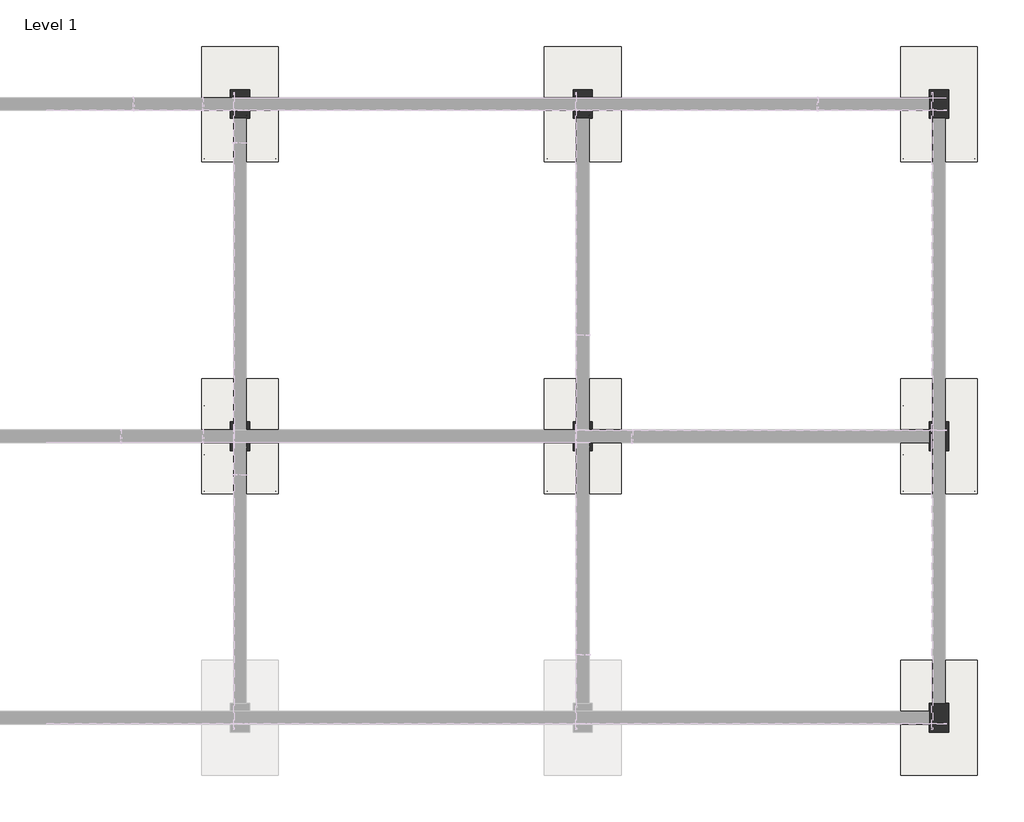
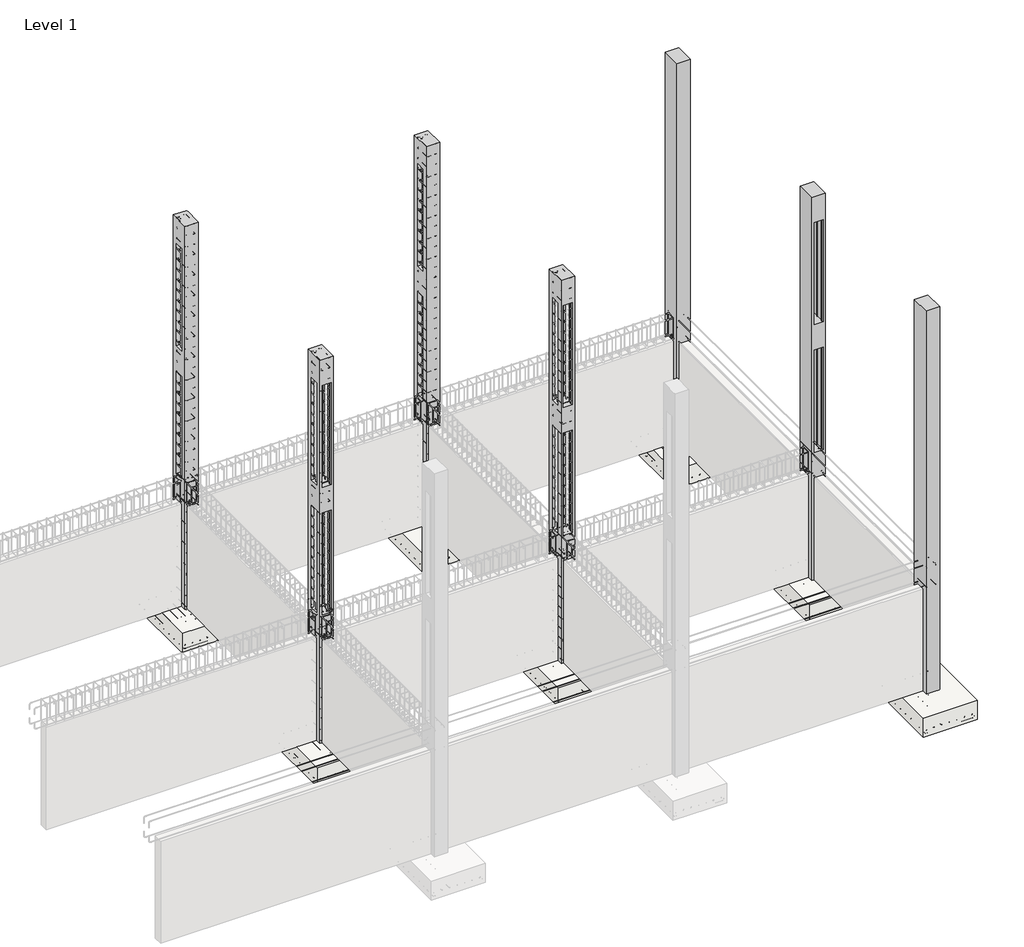
# One storey, part 2 of 8: 7 columns, 7 slabs.
"""IFC4 building model written with IfcOpenShell, lengths in millimetres."""

from ifc_helpers import new_model, si_unit, frame, origin, place, context, project, spatial, polyline, outline, extrude, faceted_brep, element, save

model = new_model("IFC4")

# Units and contexts
model_context = context("Model", 3, world=origin())
ifc_project = project(units=[si_unit("LENGTHUNIT", "METRE", prefix="MILLI")], contexts=[model_context])

# Site, building, storey
site = spatial("IfcSite", under=ifc_project)
building = spatial("IfcBuilding", under=site)
storey = spatial("IfcBuildingStorey", under=building, Name="Level 1", Elevation=0.0)

# Columns
placement = place(None, origin())
element("IfcColumn", 1, ObjectType="Concrete-Rectangular-Column : 12 x 18", at=placement, inside=storey, context=model_context, shape_type="Brep", body=[
    faceted_brep([(-14513.8601545, 13100.2555262, 0.0), (-14209.0601545, 13100.2555262, 0.0), (-14209.0601545, 12973.2555262, 0.0), (-14513.8601545, 12973.2555262, 0.0), (-14209.0601545, 13100.2555262, 9144.0), (-14209.0601545, 13024.0555262, 9144.0), (-14209.0601545, 12719.2555262, 9144.0), (-14209.0601545, 12643.0555262, 9144.0), (-14209.0601545, 12643.0555262, 0.0), (-14209.0601545, 12770.0555262, 0.0), (-14209.0601545, 12770.0555262, 2438.4), (-14209.0601545, 12973.2555262, 2438.4), (-14209.0601545, 12770.0555262, 3048.0), (-14209.0601545, 12770.0555262, 5486.4), (-14209.0601545, 12973.2555262, 5486.4), (-14209.0601545, 12973.2555262, 3048.0), (-14209.0601545, 12770.0555262, 6096.0), (-14209.0601545, 12770.0555262, 8534.4), (-14209.0601545, 12973.2555262, 8534.4), (-14209.0601545, 12973.2555262, 6096.0), (-14513.8601545, 12643.0555262, 0.0), (-14463.0601545, 12643.0555262, 0.0), (-14259.8601545, 12643.0555262, 0.0), (-14513.8601545, 12643.0555262, 9144.0), (-14513.8601545, 12719.2555262, 9144.0), (-14513.8601545, 13024.0555262, 9144.0), (-14513.8601545, 13100.2555262, 9144.0), (-14513.8601545, 12973.2555262, 2438.4), (-14513.8601545, 12770.0555262, 2438.4), (-14513.8601545, 12770.0555262, 0.0), (-14513.8601545, 12770.0555262, 5486.4), (-14513.8601545, 12770.0555262, 3048.0), (-14513.8601545, 12973.2555262, 3048.0), (-14513.8601545, 12973.2555262, 5486.4), (-14513.8601545, 12770.0555262, 8534.4), (-14513.8601545, 12770.0555262, 6096.0), (-14513.8601545, 12973.2555262, 6096.0), (-14513.8601545, 12973.2555262, 8534.4)], [[[0, 1, 2, 3]], [[4, 5, 6, 7, 8, 9, 10, 11, 2, 1], [12, 13, 14, 15], [16, 17, 18, 19]], [[20, 21, 22, 8, 7, 23]], [[20, 23, 24, 25, 26, 0, 3, 27, 28, 29], [30, 31, 32, 33], [34, 35, 36, 37]], [[1, 0, 26, 4]], [[7, 6, 5, 4, 26, 25, 24, 23]], [[9, 29, 28, 10]], [[3, 2, 11, 27]], [[11, 10, 28, 27]], [[8, 22, 21, 20, 29, 9]], [[30, 13, 12, 31]], [[32, 15, 14, 33]], [[31, 12, 15, 32]], [[13, 30, 33, 14]], [[34, 17, 16, 35]], [[36, 19, 18, 37]], [[35, 16, 19, 36]], [[17, 34, 37, 18]]]),
])
element("IfcColumn", 2, ObjectType="Concrete-Rectangular-Column : 12 x 18", at=placement, inside=storey, context=model_context, shape_type="Brep", body=[
    faceted_brep([(-9068.0732157, 13100.2555262, 0.0), (-8763.2732157, 13100.2555262, 0.0), (-8763.2732157, 12973.2555262, 0.0), (-9068.0732157, 12973.2555262, 0.0), (-8763.2732157, 13100.2555262, 9144.0), (-8763.2732157, 13024.0555262, 9144.0), (-8763.2732157, 12719.2555262, 9144.0), (-8763.2732157, 12643.0555262, 9144.0), (-8763.2732157, 12643.0555262, 0.0), (-8763.2732157, 12770.0555262, 0.0), (-8763.2732157, 12770.0555262, 2438.4), (-8763.2732157, 12973.2555262, 2438.4), (-8763.2732157, 12770.0555262, 3048.0), (-8763.2732157, 12770.0555262, 5486.4), (-8763.2732157, 12973.2555262, 5486.4), (-8763.2732157, 12973.2555262, 3048.0), (-8763.2732157, 12770.0555262, 6096.0), (-8763.2732157, 12770.0555262, 8534.4), (-8763.2732157, 12973.2555262, 8534.4), (-8763.2732157, 12973.2555262, 6096.0), (-9068.0732157, 12643.0555262, 0.0), (-9017.2732157, 12643.0555262, 0.0), (-8814.0732157, 12643.0555262, 0.0), (-9068.0732157, 12643.0555262, 9144.0), (-9068.0732157, 12719.2555262, 9144.0), (-9068.0732157, 13024.0555262, 9144.0), (-9068.0732157, 13100.2555262, 9144.0), (-9068.0732157, 12973.2555262, 2438.4), (-9068.0732157, 12770.0555262, 2438.4), (-9068.0732157, 12770.0555262, 0.0), (-9068.0732157, 12770.0555262, 5486.4), (-9068.0732157, 12770.0555262, 3048.0), (-9068.0732157, 12973.2555262, 3048.0), (-9068.0732157, 12973.2555262, 5486.4), (-9068.0732157, 12770.0555262, 8534.4), (-9068.0732157, 12770.0555262, 6096.0), (-9068.0732157, 12973.2555262, 6096.0), (-9068.0732157, 12973.2555262, 8534.4)], [[[0, 1, 2, 3]], [[4, 5, 6, 7, 8, 9, 10, 11, 2, 1], [12, 13, 14, 15], [16, 17, 18, 19]], [[20, 21, 22, 8, 7, 23]], [[20, 23, 24, 25, 26, 0, 3, 27, 28, 29], [30, 31, 32, 33], [34, 35, 36, 37]], [[1, 0, 26, 4]], [[7, 6, 5, 4, 26, 25, 24, 23]], [[9, 29, 28, 10]], [[3, 2, 11, 27]], [[11, 10, 28, 27]], [[8, 22, 21, 20, 29, 9]], [[30, 13, 12, 31]], [[32, 15, 14, 33]], [[31, 12, 15, 32]], [[13, 30, 33, 14]], [[34, 17, 16, 35]], [[36, 19, 18, 37]], [[35, 16, 19, 36]], [[17, 34, 37, 18]]]),
])
element("IfcColumn", 3, ObjectType="Concrete-Rectangular-Column : 12 x 18", at=placement, inside=storey, context=model_context, shape_type="Brep", body=[
    faceted_brep([(-3103.459716, 13100.2555262, 0.0), (-3103.459716, 12643.0555262, 0.0), (-3154.259716, 12643.0555262, 0.0), (-3357.459716, 12643.0555262, 0.0), (-3408.259716, 12643.0555262, 0.0), (-3408.259716, 12770.0555262, 0.0), (-3408.259716, 12973.2555262, 0.0), (-3408.259716, 13100.2555262, 0.0), (-3103.459716, 13100.2555262, 9144.0), (-3103.459716, 12643.0555262, 9144.0), (-3408.259716, 12643.0555262, 9144.0), (-3408.259716, 13100.2555262, 9144.0)], [[[0, 1, 2, 3, 4, 5, 6, 7]], [[8, 9, 1, 0]], [[9, 10, 4, 3, 2, 1]], [[10, 11, 7, 6, 5, 4]], [[11, 8, 0, 7]], [[8, 11, 10, 9]]]),
])
element("IfcColumn", 4, ObjectType="Concrete-Rectangular-Column : 12 x 18", at=placement, inside=storey, context=model_context, shape_type="Brep", body=[
    faceted_brep([(-3408.259716, 7364.6820829, 0.0), (-3408.259716, 7491.6820829, 0.0), (-3408.259716, 7694.8820829, 0.0), (-3408.259716, 7821.8820829, 0.0), (-3357.459716, 7821.8820829, 0.0), (-3357.459716, 7364.6820829, 0.0), (-3103.459716, 7364.6820829, 0.0), (-3103.459716, 7821.8820829, 0.0), (-3103.459716, 7821.8820829, 2438.4), (-3103.459716, 7821.8820829, 3048.0), (-3103.459716, 7821.8820829, 5486.4), (-3103.459716, 7821.8820829, 6096.0), (-3103.459716, 7821.8820829, 8534.4), (-3103.459716, 7821.8820829, 9144.0), (-3103.459716, 7364.6820829, 9144.0), (-3103.459716, 7364.6820829, 8534.4), (-3103.459716, 7364.6820829, 6096.0), (-3103.459716, 7364.6820829, 5486.4), (-3103.459716, 7364.6820829, 3048.0), (-3103.459716, 7364.6820829, 2438.4), (-3408.259716, 7364.6820829, 9144.0), (-3408.259716, 7364.6820829, 8534.4), (-3408.259716, 7364.6820829, 6096.0), (-3408.259716, 7364.6820829, 5486.4), (-3408.259716, 7364.6820829, 3048.0), (-3408.259716, 7364.6820829, 2438.4), (-3357.459716, 7364.6820829, 2438.4), (-3154.259716, 7364.6820829, 2438.4), (-3154.259716, 7364.6820829, 0.0), (-3357.459716, 7364.6820829, 3048.0), (-3357.459716, 7364.6820829, 5486.4), (-3154.259716, 7364.6820829, 5486.4), (-3154.259716, 7364.6820829, 3048.0), (-3357.459716, 7364.6820829, 6096.0), (-3357.459716, 7364.6820829, 8534.4), (-3154.259716, 7364.6820829, 8534.4), (-3154.259716, 7364.6820829, 6096.0), (-3408.259716, 7821.8820829, 9144.0), (-3408.259716, 7821.8820829, 8534.4), (-3408.259716, 7821.8820829, 6096.0), (-3408.259716, 7821.8820829, 5486.4), (-3408.259716, 7821.8820829, 3048.0), (-3408.259716, 7821.8820829, 2438.4), (-3154.259716, 7821.8820829, 0.0), (-3154.259716, 7821.8820829, 2438.4), (-3357.459716, 7821.8820829, 2438.4), (-3357.459716, 7821.8820829, 5486.4), (-3357.459716, 7821.8820829, 3048.0), (-3154.259716, 7821.8820829, 3048.0), (-3154.259716, 7821.8820829, 5486.4), (-3357.459716, 7821.8820829, 8534.4), (-3357.459716, 7821.8820829, 6096.0), (-3154.259716, 7821.8820829, 6096.0), (-3154.259716, 7821.8820829, 8534.4)], [[[0, 1, 2, 3, 4, 5]], [[6, 7, 8, 9, 10, 11, 12, 13, 14, 15, 16, 17, 18, 19]], [[6, 19, 18, 17, 16, 15, 14, 20, 21, 22, 23, 24, 25, 0, 5, 26, 27, 28], [29, 30, 31, 32], [33, 34, 35, 36]], [[3, 2, 1, 0, 25, 24, 23, 22, 21, 20, 37, 38, 39, 40, 41, 42]], [[13, 12, 11, 10, 9, 8, 7, 43, 44, 45, 4, 3, 42, 41, 40, 39, 38, 37], [46, 47, 48, 49], [50, 51, 52, 53]], [[14, 13, 37, 20]], [[5, 4, 45, 26]], [[43, 28, 27, 44]], [[27, 26, 45, 44]], [[7, 6, 28, 43]], [[46, 30, 29, 47]], [[48, 32, 31, 49]], [[47, 29, 32, 48]], [[30, 46, 49, 31]], [[50, 34, 33, 51]], [[52, 36, 35, 53]], [[51, 33, 36, 52]], [[34, 50, 53, 35]]]),
])
element("IfcColumn", 5, ObjectType="Concrete-Rectangular-Column : 12 x 18", at=placement, inside=storey, context=model_context, shape_type="Brep", body=[
    faceted_brep([(-9068.0732157, 7694.8820829, 0.0), (-9068.0732157, 7821.8820829, 0.0), (-9017.2732157, 7821.8820829, 0.0), (-9017.2732157, 7694.8820829, 0.0), (-8763.2732157, 7821.8820829, 9144.0), (-8763.2732157, 7745.6820829, 9144.0), (-8763.2732157, 7440.8820829, 9144.0), (-8763.2732157, 7364.6820829, 9144.0), (-8763.2732157, 7364.6820829, 8534.4), (-8763.2732157, 7364.6820829, 6096.0), (-8763.2732157, 7364.6820829, 5486.4), (-8763.2732157, 7364.6820829, 3048.0), (-8763.2732157, 7364.6820829, 2438.4), (-8763.2732157, 7364.6820829, 0.0), (-8763.2732157, 7491.6820829, 0.0), (-8763.2732157, 7491.6820829, 2438.4), (-8763.2732157, 7694.8820829, 2438.4), (-8763.2732157, 7694.8820829, 0.0), (-8763.2732157, 7821.8820829, 0.0), (-8763.2732157, 7821.8820829, 2438.4), (-8763.2732157, 7821.8820829, 3048.0), (-8763.2732157, 7821.8820829, 5486.4), (-8763.2732157, 7821.8820829, 6096.0), (-8763.2732157, 7821.8820829, 8534.4), (-8763.2732157, 7491.6820829, 3048.0), (-8763.2732157, 7491.6820829, 5486.4), (-8763.2732157, 7694.8820829, 5486.4), (-8763.2732157, 7694.8820829, 3048.0), (-8763.2732157, 7491.6820829, 6096.0), (-8763.2732157, 7491.6820829, 8534.4), (-8763.2732157, 7694.8820829, 8534.4), (-8763.2732157, 7694.8820829, 6096.0), (-9068.0732157, 7364.6820829, 9144.0), (-9068.0732157, 7364.6820829, 8534.4), (-9068.0732157, 7364.6820829, 6096.0), (-9068.0732157, 7364.6820829, 5486.4), (-9068.0732157, 7364.6820829, 3048.0), (-9068.0732157, 7364.6820829, 2438.4), (-9068.0732157, 7364.6820829, 0.0), (-9017.2732157, 7364.6820829, 0.0), (-9017.2732157, 7364.6820829, 2438.4), (-8814.0732157, 7364.6820829, 2438.4), (-8814.0732157, 7364.6820829, 0.0), (-9017.2732157, 7364.6820829, 3048.0), (-9017.2732157, 7364.6820829, 5486.4), (-8814.0732157, 7364.6820829, 5486.4), (-8814.0732157, 7364.6820829, 3048.0), (-9017.2732157, 7364.6820829, 6096.0), (-9017.2732157, 7364.6820829, 8534.4), (-8814.0732157, 7364.6820829, 8534.4), (-8814.0732157, 7364.6820829, 6096.0), (-9068.0732157, 7440.8820829, 9144.0), (-9068.0732157, 7745.6820829, 9144.0), (-9068.0732157, 7821.8820829, 9144.0), (-9068.0732157, 7821.8820829, 8534.4), (-9068.0732157, 7821.8820829, 6096.0), (-9068.0732157, 7821.8820829, 5486.4), (-9068.0732157, 7821.8820829, 3048.0), (-9068.0732157, 7821.8820829, 2438.4), (-9068.0732157, 7694.8820829, 2438.4), (-9068.0732157, 7491.6820829, 2438.4), (-9068.0732157, 7491.6820829, 0.0), (-9068.0732157, 7491.6820829, 5486.4), (-9068.0732157, 7491.6820829, 3048.0), (-9068.0732157, 7694.8820829, 3048.0), (-9068.0732157, 7694.8820829, 5486.4), (-9068.0732157, 7491.6820829, 8534.4), (-9068.0732157, 7491.6820829, 6096.0), (-9068.0732157, 7694.8820829, 6096.0), (-9068.0732157, 7694.8820829, 8534.4), (-8814.0732157, 7821.8820829, 0.0), (-8814.0732157, 7821.8820829, 2438.4), (-9017.2732157, 7821.8820829, 2438.4), (-9017.2732157, 7821.8820829, 5486.4), (-9017.2732157, 7821.8820829, 3048.0), (-8814.0732157, 7821.8820829, 3048.0), (-8814.0732157, 7821.8820829, 5486.4), (-9017.2732157, 7821.8820829, 8534.4), (-9017.2732157, 7821.8820829, 6096.0), (-8814.0732157, 7821.8820829, 6096.0), (-8814.0732157, 7821.8820829, 8534.4), (-9017.2732157, 7491.6820829, 2438.4), (-9017.2732157, 7491.6820829, 0.0), (-8814.0732157, 7694.8820829, 2438.4), (-8814.0732157, 7694.8820829, 0.0), (-8814.0732157, 7491.6820829, 2438.4), (-9017.2732157, 7694.8820829, 2438.4), (-8814.0732157, 7491.6820829, 0.0), (-9017.2732157, 7491.6820829, 5486.4), (-9017.2732157, 7491.6820829, 3048.0), (-8814.0732157, 7694.8820829, 5486.4), (-8814.0732157, 7694.8820829, 3048.0), (-9017.2732157, 7694.8820829, 3048.0), (-8814.0732157, 7491.6820829, 3048.0), (-8814.0732157, 7491.6820829, 5486.4), (-9017.2732157, 7694.8820829, 5486.4), (-9017.2732157, 7491.6820829, 8534.4), (-9017.2732157, 7491.6820829, 6096.0), (-8814.0732157, 7694.8820829, 8534.4), (-8814.0732157, 7694.8820829, 6096.0), (-9017.2732157, 7694.8820829, 6096.0), (-8814.0732157, 7491.6820829, 6096.0), (-8814.0732157, 7491.6820829, 8534.4), (-9017.2732157, 7694.8820829, 8534.4)], [[[0, 1, 2, 3]], [[4, 5, 6, 7, 8, 9, 10, 11, 12, 13, 14, 15, 16, 17, 18, 19, 20, 21, 22, 23], [24, 25, 26, 27], [28, 29, 30, 31]], [[13, 12, 11, 10, 9, 8, 7, 32, 33, 34, 35, 36, 37, 38, 39, 40, 41, 42], [43, 44, 45, 46], [47, 48, 49, 50]], [[38, 37, 36, 35, 34, 33, 32, 51, 52, 53, 54, 55, 56, 57, 58, 1, 0, 59, 60, 61], [62, 63, 64, 65], [66, 67, 68, 69]], [[4, 23, 22, 21, 20, 19, 18, 70, 71, 72, 2, 1, 58, 57, 56, 55, 54, 53], [73, 74, 75, 76], [77, 78, 79, 80]], [[7, 6, 5, 4, 53, 52, 51, 32]], [[61, 60, 81, 82]], [[17, 16, 83, 84]], [[16, 15, 85, 41, 40, 81, 60, 59, 86, 72, 71, 83]], [[38, 61, 82, 39]], [[3, 2, 72, 86]], [[42, 41, 85, 87]], [[18, 17, 84, 70]], [[14, 13, 42, 87]], [[40, 39, 82, 81]], [[70, 84, 83, 71]], [[15, 14, 87, 85]], [[59, 0, 3, 86]], [[63, 62, 88, 89]], [[27, 26, 90, 91]], [[24, 27, 91, 75, 74, 92, 64, 63, 89, 43, 46, 93]], [[26, 25, 94, 45, 44, 88, 62, 65, 95, 73, 76, 90]], [[73, 95, 92, 74]], [[93, 46, 45, 94]], [[25, 24, 93, 94]], [[65, 64, 92, 95]], [[88, 44, 43, 89]], [[75, 91, 90, 76]], [[67, 66, 96, 97]], [[31, 30, 98, 99]], [[28, 31, 99, 79, 78, 100, 68, 67, 97, 47, 50, 101]], [[30, 29, 102, 49, 48, 96, 66, 69, 103, 77, 80, 98]], [[77, 103, 100, 78]], [[101, 50, 49, 102]], [[29, 28, 101, 102]], [[69, 68, 100, 103]], [[96, 48, 47, 97]], [[79, 99, 98, 80]]]),
])
element("IfcColumn", 6, ObjectType="Concrete-Rectangular-Column : 12 x 18", at=placement, inside=storey, context=model_context, shape_type="Brep", body=[
    faceted_brep([(-14513.8601545, 7694.8820829, 0.0), (-14513.8601545, 7821.8820829, 0.0), (-14463.0601545, 7821.8820829, 0.0), (-14463.0601545, 7694.8820829, 0.0), (-14209.0601545, 7821.8820829, 9144.0), (-14209.0601545, 7745.6820829, 9144.0), (-14209.0601545, 7440.8820829, 9144.0), (-14209.0601545, 7364.6820829, 9144.0), (-14209.0601545, 7364.6820829, 8534.4), (-14209.0601545, 7364.6820829, 6096.0), (-14209.0601545, 7364.6820829, 5486.4), (-14209.0601545, 7364.6820829, 3048.0), (-14209.0601545, 7364.6820829, 2438.4), (-14209.0601545, 7364.6820829, 0.0), (-14209.0601545, 7491.6820829, 0.0), (-14209.0601545, 7491.6820829, 2438.4), (-14209.0601545, 7694.8820829, 2438.4), (-14209.0601545, 7694.8820829, 0.0), (-14209.0601545, 7821.8820829, 0.0), (-14209.0601545, 7821.8820829, 2438.4), (-14209.0601545, 7821.8820829, 3048.0), (-14209.0601545, 7821.8820829, 5486.4), (-14209.0601545, 7821.8820829, 6096.0), (-14209.0601545, 7821.8820829, 8534.4), (-14209.0601545, 7491.6820829, 3048.0), (-14209.0601545, 7491.6820829, 5486.4), (-14209.0601545, 7694.8820829, 5486.4), (-14209.0601545, 7694.8820829, 3048.0), (-14209.0601545, 7491.6820829, 6096.0), (-14209.0601545, 7491.6820829, 8534.4), (-14209.0601545, 7694.8820829, 8534.4), (-14209.0601545, 7694.8820829, 6096.0), (-14513.8601545, 7364.6820829, 9144.0), (-14513.8601545, 7364.6820829, 8534.4), (-14513.8601545, 7364.6820829, 6096.0), (-14513.8601545, 7364.6820829, 5486.4), (-14513.8601545, 7364.6820829, 3048.0), (-14513.8601545, 7364.6820829, 2438.4), (-14513.8601545, 7364.6820829, 0.0), (-14463.0601545, 7364.6820829, 0.0), (-14463.0601545, 7364.6820829, 2438.4), (-14259.8601545, 7364.6820829, 2438.4), (-14259.8601545, 7364.6820829, 0.0), (-14259.8601545, 7364.6820829, 5486.4), (-14259.8601545, 7364.6820829, 3048.0), (-14463.0601545, 7364.6820829, 3048.0), (-14463.0601545, 7364.6820829, 5486.4), (-14259.8601545, 7364.6820829, 8534.4), (-14259.8601545, 7364.6820829, 6096.0), (-14463.0601545, 7364.6820829, 6096.0), (-14463.0601545, 7364.6820829, 8534.4), (-14513.8601545, 7440.8820829, 9144.0), (-14513.8601545, 7745.6820829, 9144.0), (-14513.8601545, 7821.8820829, 9144.0), (-14513.8601545, 7821.8820829, 8534.4), (-14513.8601545, 7821.8820829, 6096.0), (-14513.8601545, 7821.8820829, 5486.4), (-14513.8601545, 7821.8820829, 3048.0), (-14513.8601545, 7821.8820829, 2438.4), (-14513.8601545, 7694.8820829, 2438.4), (-14513.8601545, 7491.6820829, 2438.4), (-14513.8601545, 7491.6820829, 0.0), (-14513.8601545, 7491.6820829, 5486.4), (-14513.8601545, 7491.6820829, 3048.0), (-14513.8601545, 7694.8820829, 3048.0), (-14513.8601545, 7694.8820829, 5486.4), (-14513.8601545, 7491.6820829, 8534.4), (-14513.8601545, 7491.6820829, 6096.0), (-14513.8601545, 7694.8820829, 6096.0), (-14513.8601545, 7694.8820829, 8534.4), (-14259.8601545, 7821.8820829, 0.0), (-14259.8601545, 7821.8820829, 2438.4), (-14463.0601545, 7821.8820829, 2438.4), (-14259.8601545, 7821.8820829, 3048.0), (-14259.8601545, 7821.8820829, 5486.4), (-14463.0601545, 7821.8820829, 5486.4), (-14463.0601545, 7821.8820829, 3048.0), (-14259.8601545, 7821.8820829, 6096.0), (-14259.8601545, 7821.8820829, 8534.4), (-14463.0601545, 7821.8820829, 8534.4), (-14463.0601545, 7821.8820829, 6096.0), (-14463.0601545, 7491.6820829, 2438.4), (-14463.0601545, 7491.6820829, 0.0), (-14259.8601545, 7694.8820829, 2438.4), (-14259.8601545, 7694.8820829, 0.0), (-14259.8601545, 7491.6820829, 2438.4), (-14463.0601545, 7694.8820829, 2438.4), (-14259.8601545, 7491.6820829, 0.0), (-14463.0601545, 7491.6820829, 5486.4), (-14463.0601545, 7491.6820829, 3048.0), (-14259.8601545, 7694.8820829, 5486.4), (-14259.8601545, 7694.8820829, 3048.0), (-14463.0601545, 7694.8820829, 3048.0), (-14259.8601545, 7491.6820829, 3048.0), (-14259.8601545, 7491.6820829, 5486.4), (-14463.0601545, 7694.8820829, 5486.4), (-14463.0601545, 7491.6820829, 8534.4), (-14463.0601545, 7491.6820829, 6096.0), (-14259.8601545, 7694.8820829, 8534.4), (-14259.8601545, 7694.8820829, 6096.0), (-14463.0601545, 7694.8820829, 6096.0), (-14259.8601545, 7491.6820829, 6096.0), (-14259.8601545, 7491.6820829, 8534.4), (-14463.0601545, 7694.8820829, 8534.4)], [[[0, 1, 2, 3]], [[4, 5, 6, 7, 8, 9, 10, 11, 12, 13, 14, 15, 16, 17, 18, 19, 20, 21, 22, 23], [24, 25, 26, 27], [28, 29, 30, 31]], [[13, 12, 11, 10, 9, 8, 7, 32, 33, 34, 35, 36, 37, 38, 39, 40, 41, 42], [43, 44, 45, 46], [47, 48, 49, 50]], [[38, 37, 36, 35, 34, 33, 32, 51, 52, 53, 54, 55, 56, 57, 58, 1, 0, 59, 60, 61], [62, 63, 64, 65], [66, 67, 68, 69]], [[4, 23, 22, 21, 20, 19, 18, 70, 71, 72, 2, 1, 58, 57, 56, 55, 54, 53], [73, 74, 75, 76], [77, 78, 79, 80]], [[7, 6, 5, 4, 53, 52, 51, 32]], [[61, 60, 81, 82]], [[17, 16, 83, 84]], [[16, 15, 85, 41, 40, 81, 60, 59, 86, 72, 71, 83]], [[38, 61, 82, 39]], [[42, 41, 85, 87]], [[3, 2, 72, 86]], [[18, 17, 84, 70]], [[15, 14, 87, 85]], [[59, 0, 3, 86]], [[14, 13, 42, 87]], [[70, 84, 83, 71]], [[40, 39, 82, 81]], [[63, 62, 88, 89]], [[27, 26, 90, 91]], [[24, 27, 91, 73, 76, 92, 64, 63, 89, 45, 44, 93]], [[26, 25, 94, 43, 46, 88, 62, 65, 95, 75, 74, 90]], [[43, 94, 93, 44]], [[92, 76, 75, 95]], [[25, 24, 93, 94]], [[65, 64, 92, 95]], [[90, 74, 73, 91]], [[45, 89, 88, 46]], [[67, 66, 96, 97]], [[31, 30, 98, 99]], [[28, 31, 99, 77, 80, 100, 68, 67, 97, 49, 48, 101]], [[30, 29, 102, 47, 50, 96, 66, 69, 103, 79, 78, 98]], [[47, 102, 101, 48]], [[100, 80, 79, 103]], [[29, 28, 101, 102]], [[69, 68, 100, 103]], [[98, 78, 77, 99]], [[49, 97, 96, 50]]]),
])
element("IfcColumn", 7, ObjectType="Concrete-Rectangular-Column : 12 x 18", at=placement, inside=storey, context=model_context, shape_type="Brep", body=[
    faceted_brep([(-3103.459716, 3351.1050327, 0.0), (-3103.459716, 2893.9050327, 0.0), (-3408.259716, 2893.9050327, 0.0), (-3408.259716, 3020.9050327, 0.0), (-3408.259716, 3224.1050327, 0.0), (-3408.259716, 3351.1050327, 0.0), (-3357.459716, 3351.1050327, 0.0), (-3154.259716, 3351.1050327, 0.0), (-3103.459716, 3351.1050327, 9144.0), (-3103.459716, 2893.9050327, 9144.0), (-3408.259716, 2893.9050327, 9144.0), (-3408.259716, 3351.1050327, 9144.0)], [[[0, 1, 2, 3, 4, 5, 6, 7]], [[8, 9, 1, 0]], [[9, 10, 2, 1]], [[10, 11, 5, 4, 3, 2]], [[11, 8, 0, 7, 6, 5]], [[8, 11, 10, 9]]]),
])

# Slabs
element("IfcSlab", 8, ObjectType="Footing-Rectangular : 72\" x 48\" x 18\"", at=placement, inside=storey, context=model_context, shape_type="SweptSolid", body=[
    extrude(outline(polyline([(-13751.8601545, 13786.0555262), (-13751.8601545, 11957.2555262), (-14971.0601545, 11957.2555262), (-14971.0601545, 13786.0555262), (-13751.8601545, 13786.0555262)])), frame((0.0, 0.0, -457.2), z_axis=(0.0, 0.0, 1.0), x_axis=(1.0, 0.0, 0.0)), (0.0, 0.0, 1.0), 457.2),
])
element("IfcSlab", 9, ObjectType="Footing-Rectangular : 72\" x 48\" x 18\"", at=placement, inside=storey, context=model_context, shape_type="SweptSolid", body=[
    extrude(outline(polyline([(-8306.0732157, 13786.0555262), (-8306.0732157, 11957.2555262), (-9525.2732157, 11957.2555262), (-9525.2732157, 13786.0555262), (-8306.0732157, 13786.0555262)])), frame((0.0, 0.0, -457.2), z_axis=(0.0, 0.0, 1.0), x_axis=(1.0, 0.0, 0.0)), (0.0, 0.0, 1.0), 457.2),
])
element("IfcSlab", 10, ObjectType="Footing-Rectangular : 72\" x 48\" x 18\"", at=placement, inside=storey, context=model_context, shape_type="SweptSolid", body=[
    extrude(outline(polyline([(-2646.259716, 13786.0555262), (-2646.259716, 11957.2555262), (-3865.459716, 11957.2555262), (-3865.459716, 13786.0555262), (-2646.259716, 13786.0555262)])), frame((0.0, 0.0, -457.2), z_axis=(0.0, 0.0, 1.0), x_axis=(1.0, 0.0, 0.0)), (0.0, 0.0, 1.0), 457.2),
])
element("IfcSlab", 11, ObjectType="Footing-Rectangular : 72\" x 48\" x 18\"", at=placement, inside=storey, context=model_context, shape_type="SweptSolid", body=[
    extrude(outline(polyline([(-2646.259716, 8507.6820829), (-2646.259716, 6678.8820829), (-3865.459716, 6678.8820829), (-3865.459716, 8507.6820829), (-2646.259716, 8507.6820829)])), frame((0.0, 0.0, -457.2), z_axis=(0.0, 0.0, 1.0), x_axis=(1.0, 0.0, 0.0)), (0.0, 0.0, 1.0), 457.2),
])
element("IfcSlab", 12, ObjectType="Footing-Rectangular : 72\" x 48\" x 18\"", at=placement, inside=storey, context=model_context, shape_type="SweptSolid", body=[
    extrude(outline(polyline([(-8306.0732157, 8507.6820829), (-8306.0732157, 6678.8820829), (-9525.2732157, 6678.8820829), (-9525.2732157, 8507.6820829), (-8306.0732157, 8507.6820829)])), frame((0.0, 0.0, -457.2), z_axis=(0.0, 0.0, 1.0), x_axis=(1.0, 0.0, 0.0)), (0.0, 0.0, 1.0), 457.2),
])
element("IfcSlab", 13, ObjectType="Footing-Rectangular : 72\" x 48\" x 18\"", at=placement, inside=storey, context=model_context, shape_type="SweptSolid", body=[
    extrude(outline(polyline([(-13751.8601545, 8507.6820829), (-13751.8601545, 6678.8820829), (-14971.0601545, 6678.8820829), (-14971.0601545, 8507.6820829), (-13751.8601545, 8507.6820829)])), frame((0.0, 0.0, -457.2), z_axis=(0.0, 0.0, 1.0), x_axis=(1.0, 0.0, 0.0)), (0.0, 0.0, 1.0), 457.2),
])
element("IfcSlab", 14, ObjectType="Footing-Rectangular : 72\" x 48\" x 18\"", at=placement, inside=storey, context=model_context, shape_type="SweptSolid", body=[
    extrude(outline(polyline([(-2646.259716, 4036.9050327), (-2646.259716, 2208.1050327), (-3865.459716, 2208.1050327), (-3865.459716, 4036.9050327), (-2646.259716, 4036.9050327)])), frame((0.0, 0.0, -457.2), z_axis=(0.0, 0.0, 1.0), x_axis=(1.0, 0.0, 0.0)), (0.0, 0.0, 1.0), 457.2),
])

save(model, "model.ifc")

# Revit data of these elements
# Type "Concrete-Rectangular-Column : 12 x 18"
#   Assembly Code = "B10"
#   b = 1' - 0"
#   h = 1' - 6"
#   Structural Material [instance default] = Concrete, Cast-in-Place gray
# Type "Footing-Rectangular : 72\" x 48\" x 18\""
#   Assembly Code = "A1010100"
#   Width = 4' - 0"
#   Length = 6' - 0"
#   Foundation Thickness = 1' - 6"
#   Structural Material [instance default] = Concrete, Cast-in-Place gray
# Elements 1, 2, 3, 4, 5, 6, 7 (IfcColumn, "Concrete-Rectangular-Column : 12 x 18")
#   Structural Material = Concrete, Cast-in-Place gray
#   Phase Created = New Construction
#   Materials on its faces: "Concrete, Cast-in-Place gray"
# Elements 8, 9, 10, 11, 12, 13, 14 (IfcSlab, "Footing-Rectangular : 72\" x 48\" x 18\"")
#   Structural Material = Concrete, Cast-in-Place gray
#   Phase Created = New Construction
#   Materials on its faces: "Concrete, Cast-in-Place gray"
# Materials
#   "Concrete, Cast-in-Place gray": class "Concrete", colour RGB 192 192 192, transparency 0, Description = "Cast-in-place concrete", Cost = 0
